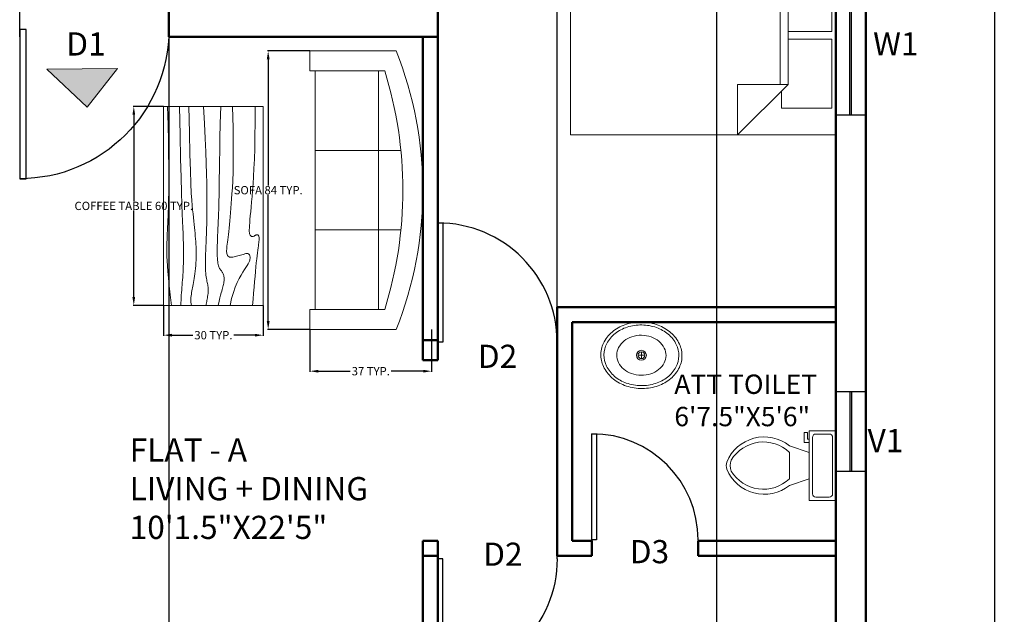
# Model space of a CAD drawing. Units: inches. Extents: x 227 to 711, y 218 to 1048.
# Tile 3 of 5: x 414 to 711, y 411 to 590. Entities that reach past the tile are written whole.
import ezdxf

# ---------------------------------------------------------------- set-up
doc = ezdxf.new("R2010")
doc.units = ezdxf.units.IN
doc.header["$MEASUREMENT"] = 0
for name, color, linetype, lineweight in [('A-ANNO-DIMS', 2, 'Continuous', 18), ('A-ANNO-SYMB', 85, 'Continuous', 18), ('A-ANNO-TEXT', 70, 'Continuous', 18), ('A-AREA-IDEN', 70, 'Continuous', 25), ('A-FLOR-FIXT', 140, 'Continuous', 18), ('A-FURN', 8, 'Continuous', 18), ('A-WALL', 10, 'Continuous', 50), ('DOORS', 30, 'Continuous', 25), ('WINDOWS', 50, 'Continuous', 25)]:
    doc.layers.add(name, color=color, linetype=linetype, lineweight=lineweight)
doc.styles.get("Standard").update_dxf_attribs({"font": 'arial.ttf'})
doc.dimstyles.get("Standard").update_dxf_attribs({"dimtxt": 2.5, "dimasz": 2.5, "dimexe": 0.18, "dimexo": 0.0625, "dimgap": 0.09, "dimtad": 0, "dimtih": 1, "dimtoh": 1, "dimzin": 0, "dimdsep": 46, "dimlunit": 3, "dimtxsty": 'Standard', "dimcen": 0.09, "dimadec": 0, "dimazin": 0, "dimtfac": 1, "dimtofl": 0, "dimtmove": 0, "dimatfit": 3, "dimfxl": 1, "dimtolj": 1, "dimtzin": 0, "dimarcsym": 0})

# ---------------------------------------------------------------- blocks, each defined once
blk = doc.blocks.new('*U2')
for p, q in [((0, 0), (0, -6)), ((40, 0), (40, -6))]:
    blk.add_line(p, q)
blk.add_lwpolyline([(0, 0), (0, 40), (1.75, 40), (1.75, 0)], close=True)
blk.add_arc((0, 0), 40, 0, 90)
blk = doc.blocks.new('Bed - Queen')
for p, q in [((0, -80.00003), (0, 0)), ((0, 0), (59.99999, 0)), ((59.99999, 0), (59.99999, -80.00003)), ((7.99999, -1.2), (28.79998, -1.2)), ((7.99999, -14.4), (7.99999, -1.2)), ((28.79998, -1.2), (28.79998, -14.4)), ((31.19999, -1.2), (51.99999, -1.2)), ((31.19999, -14.4), (31.19999, -1.2)), ((51.99999, -1.2), (51.99999, -16.4)), ((0, -14.4), (44.8, -14.4)), ((59.99999, -29.6), (44.8, -14.4)), ((44.8, -14.4), (44.8, -29.6)), ((44.8, -16.8), (0, -16.8)), ((51.99999, -16.4), (46.79936, -16.4)), ((44.8, -29.6), (59.99999, -29.6)), ((59.99999, -80.00003), (0, -80.00003))]:
    blk.add_line(p, q)
blk = doc.blocks.new('Toilet - top')
for p, q in [((9.5, -6), (9.5, -2)), ((-10, -8.5), (-8, -8.5)), ((-10, -9.5), (-10, -8.5)), ((-8, -8.5), (-8, -8)), ((-7, -8), (-7, -9.5)), ((-4, -8), (-6, -14)), ((4, -8), (6, -14)), ((-7, -9.5), (-10, -9.5)), ((4, -14), (-4, -14))]:
    blk.add_line(p, q)
blk.add_lwpolyline([(10.5, -8), (10.5, 0), (-10.5, 0), (-10.5, -8)], close=True)
for points in [[(-9.5, -2), (-9.5, -6)], [(8.5, -1), (-8.5, -1)], [(-8.5, -7), (8.5, -7)]]:
    blk.add_lwpolyline(points)
for centre, radius, start, end in [((-8.62, -1.88), 0.884, 81.8699, 188.1301), ((8.62, -1.88), 0.884, 351.8699, 98.1301), ((-8.62, -6.12), 0.884, 171.8699, 278.1301), ((8.62, -6.12), 0.884, 261.8699, 8.1301), ((3.52, -21.58), 12.17, 141.4691, 247.9714), ((4.2, -21.82), 11.33, 136.3677, 238.9468), ((-3.52, -21.58), 12.17, 292.0284, 38.5307), ((-4.2, -21.82), 11.33, 301.053, 43.6321), ((0, -27.88), 4, 245.7318, 294.2682), ((0, -29), 4, 254.8605, 285.1395)]:
    blk.add_arc(centre, radius, start, end)
blk = doc.blocks.new('Sink - Oval top')
for p, q in [((-1, 0), (1, 0)), ((0, 1), (0, -1))]:
    blk.add_line(p, q)
for points in [[(-12.23, 0.39, 0.117634), (-11.46, -3.36, 0.104469), (-8.88, -6.8, 0.090016), (-5.08, -9.07, 0.08192), (-0.32, -10.02, 0.08192), (4.49, -9.38, 0.090016), (8.42, -7.36, 0.104469), (11.22, -4.09, 0.117634), (12.23, -0.39, 0.117634), (11.46, 3.36, 0.104469), (8.88, 6.8, 0.090016), (5.08, 9.07, 0.08192), (0.32, 10.02, 0.08192), (-4.49, 9.38, 0.090016), (-8.42, 7.36, 0.104469), (-11.22, 4.09, 0.117634)], [(-11.29, 0.16, 0.118622), (-10.52, -3.25, 0.104678), (-8.07, -6.36, 0.089562), (-4.54, -8.37, 0.081185), (-0.13, -9.15, 0.081185), (4.3, -8.49, 0.089562), (7.89, -6.58, 0.104678), (10.42, -3.55, 0.118622), (11.29, -0.16, 0.118622), (10.52, 3.25, 0.104678), (8.07, 6.36, 0.089562), (4.54, 8.37, 0.081185), (0.13, 9.15, 0.081185), (-4.3, 8.49, 0.089562), (-7.89, 6.58, 0.104678), (-10.42, 3.55, 0.118622)], [(-7.42, 0.08, 0.118283), (-6.91, -2.17, 0.104607), (-5.29, -4.21, 0.089718), (-2.97, -5.53, 0.081436), (-0.07, -6.04, 0.081436), (2.84, -5.59, 0.089718), (5.2, -4.33, 0.104607), (6.86, -2.32, 0.118283), (7.42, -0.08, 0.118283), (6.91, 2.17, 0.104607), (5.29, 4.21, 0.089718), (2.97, 5.53, 0.081436), (0.07, 6.04, 0.081436), (-2.84, 5.59, 0.089718), (-5.2, 4.33, 0.104607), (-6.86, 2.32, 0.118283)]]:
    blk.add_lwpolyline(points, format="xyb", close=True)
for radius in [1.5, 1]:
    blk.add_circle((0, 0), radius)
blk = doc.blocks.new('Sofa - Roundback 7 ft.')
for p, q in [((-12.00002, -32.4421), (-12.00003, -6.5971)), ((11.99997, -32.4421), (11.99998, -6.5971)), ((-36.000027, -34), (-36.000027, -11.4696)), ((35.99998, -34), (35.99998, -11.4696)), ((-35.999844, -13.3819), (35.9998, -13.3819)), ((-36.000027, -32.4421), (35.99998, -32.4421))]:
    blk.add_line(p, q)
for points in [[(-36.000027, -34), (-42.000027, -34), (-42.000027, -8)], [(41.99998, -8), (41.99998, -34), (35.99998, -34)]]:
    blk.add_lwpolyline(points)
for centre, radius, start, end in [((0, -114.25), 114.25, 68.43141, 111.5686), ((-0.00001, -127.1968), 121.1968, 72.72033, 107.2797)]:
    blk.add_arc(centre, radius, start, end)
blk = doc.blocks.new('Table - Rectangular Woodgrain 60 x 30 in.')
for p, q in [((0, 0), (0, -30)), ((60, 0), (0, 0)), ((60, -30), (60, 0)), ((0, -30), (60, -30))]:
    blk.add_line(p, q)
for points in [[(0, -2.4), (4.8155, -2.418), (9.0302, -2.4688), (12.709, -2.5477), (15.9167, -2.65), (18.7181, -2.7711), (21.1781, -2.9063), (23.3616, -3.0508), (25.3333, -3.2), (27.1477, -3.3495), (28.8172, -3.4958), (30.3437, -3.636), (31.7291, -3.7667), (32.9756, -3.8849), (34.0849, -3.9875), (35.059, -4.0714), (35.9, -4.1334), (36.6114, -4.1711), (37.2041, -4.1854), (37.6906, -4.1779), (38.0833, -4.15), (38.3948, -4.1034), (38.6375, -4.0396), (38.8239, -3.9602), (38.9666, -3.8667), (39.0764, -3.7608), (39.1573, -3.6448), (39.2116, -3.521), (39.2416, -3.3917), (39.2498, -3.2593), (39.2385, -3.1261), (39.21, -2.9944), (39.1666, -2.8667), (39.111, -2.7447), (39.0468, -2.6281), (38.978, -2.5163), (38.9083, -2.4083), (38.8418, -2.3035), (38.7823, -2.201), (38.7337, -2.1001), (38.7, -2), (38.6844, -1.9003), (38.6875, -1.8021), (38.7094, -1.707), (38.75, -1.6167), (38.8094, -1.5326), (38.8875, -1.4563), (38.9844, -1.3893), (39.1, -1.3333), (39.2351, -1.2896), (39.3937, -1.2583), (39.5804, -1.2396), (39.8, -1.2333), (40.057, -1.2396), (40.3562, -1.2583), (40.7023, -1.2896), (41.1, -1.3333), (41.5547, -1.3895), (42.0755, -1.4573), (42.6721, -1.5361), (43.3542, -1.625), (44.1316, -1.7233), (45.014, -1.8302), (46.0114, -1.9449), (47.1333, -2.0667), (48.3862, -2.1947), (49.7625, -2.3281), (51.2513, -2.4663), (52.8416, -2.6083), (54.5226, -2.7535), (56.2833, -2.9011), (58.1127, -3.0501), (60, -3.2)], [(0, -9.2), (6.5759, -9.0858), (11.9385, -9.0365), (16.2527, -9.0418), (19.6833, -9.0917), (22.3952, -9.1759), (24.5531, -9.2844), (26.322, -9.4069), (27.8666, -9.5333), (29.3241, -9.6553), (30.7203, -9.7719), (32.0532, -9.8837), (33.3208, -9.9917), (34.5213, -10.0965), (35.6526, -10.199), (36.7128, -10.2999), (37.7, -10.4), (38.6129, -10.4996), (39.4531, -10.5969), (40.223, -10.6895), (40.925, -10.775), (41.5613, -10.8512), (42.1344, -10.9156), (42.6465, -10.966), (43.1, -11), (43.4976, -11.0158), (43.8437, -11.0136), (44.143, -10.9942), (44.4, -10.9583), (44.6195, -10.9069), (44.8062, -10.8406), (44.9648, -10.7603), (45.1, -10.6667), (45.2155, -10.5598), (45.3114, -10.4365), (45.3871, -10.2929), (45.4416, -10.125), (45.4743, -9.929), (45.4844, -9.7011), (45.4709, -9.4371), (45.4333, -9.1333), (45.3716, -8.7883), (45.2896, -8.4104), (45.1919, -8.0107), (45.0833, -7.6), (44.9685, -7.1893), (44.8521, -6.7896), (44.7388, -6.4117), (44.6333, -6.0667), (44.54, -5.7628), (44.4614, -5.4979), (44.4001, -5.2675), (44.3583, -5.0667), (44.3384, -4.8909), (44.3427, -4.7354), (44.3736, -4.5956), (44.4333, -4.4667), (44.5236, -4.3453), (44.6427, -4.2333), (44.7884, -4.1339), (44.9583, -4.05), (45.1501, -3.9849), (45.3614, -3.9417), (45.59, -3.9234), (45.8333, -3.9333), (46.0915, -3.9749), (46.3734, -4.0531), (46.6906, -4.1736), (47.0542, -4.3417), (47.4756, -4.5629), (47.9661, -4.8427), (48.5372, -5.1866), (49.2, -5.6), (49.9676, -6.0844), (50.8594, -6.625), (51.8965, -7.2031), (53.1, -7.8), (54.491, -8.3969), (56.0906, -8.975), (57.9199, -9.5156), (60, -10)], [(0, -12.8), (5.1847, -12.9322), (9.6213, -13.0323), (13.3963, -13.1059), (16.5958, -13.1583), (19.3063, -13.1952), (21.614, -13.2219), (23.6054, -13.2439), (25.3666, -13.2667), (26.9728, -13.2947), (28.4531, -13.3281), (29.8256, -13.3663), (31.1083, -13.4083), (32.3191, -13.4535), (33.476, -13.501), (34.597, -13.5501), (35.7, -13.6), (36.7984, -13.6497), (37.8875, -13.6979), (38.9578, -13.743), (40, -13.7833), (41.0047, -13.8174), (41.9625, -13.8438), (42.864, -13.8607), (43.7, -13.8667), (44.4631, -13.8604), (45.1552, -13.8417), (45.7801, -13.8104), (46.3416, -13.7667), (46.8439, -13.7104), (47.2906, -13.6417), (47.6858, -13.5604), (48.0333, -13.4667), (48.3375, -13.3608), (48.6042, -13.2448), (48.8396, -13.121), (49.05, -12.9917), (49.2417, -12.8593), (49.4208, -12.7261), (49.5937, -12.5944), (49.7667, -12.4667), (49.9452, -12.3451), (50.1323, -12.2313), (50.3303, -12.1268), (50.5416, -12.0333), (50.7686, -11.9524), (51.0135, -11.8854), (51.2788, -11.8341), (51.5666, -11.8), (51.8785, -11.7843), (52.2116, -11.7865), (52.562, -11.8059), (52.926, -11.8417), (53.2998, -11.8931), (53.6795, -11.9594), (54.0614, -12.0397), (54.4416, -12.1333), (54.8223, -12.2401), (55.2293, -12.3625), (55.6942, -12.5037), (56.2489, -12.6667), (56.9251, -12.8547), (57.7545, -13.0708), (58.7689, -13.3182), (60, -13.6)], [(0, -18), (5.124, -17.7273), (9.6609, -17.5057), (13.6705, -17.3303), (17.2125, -17.1958), (20.3467, -17.0973), (23.1328, -17.0297), (25.6307, -16.9878), (27.9, -16.9667), (29.9928, -16.9617), (31.9302, -16.9703), (33.7254, -16.9907), (35.3917, -17.0208), (36.9423, -17.0588), (38.3906, -17.1026), (39.7499, -17.1503), (41.0333, -17.2), (42.2519, -17.2496), (43.4073, -17.2969), (44.4986, -17.3395), (45.525, -17.375), (46.4858, -17.4012), (47.3802, -17.4156), (48.2074, -17.416), (48.9667, -17.4), (49.6583, -17.3662), (50.2872, -17.3167), (50.8595, -17.2547), (51.3812, -17.1833), (51.8584, -17.1057), (52.2971, -17.025), (52.7034, -16.9443), (53.0833, -16.8667), (53.443, -16.7951), (53.789, -16.7313), (54.128, -16.6768), (54.4666, -16.6334), (54.8115, -16.6024), (55.1693, -16.5854), (55.5465, -16.5841), (55.95, -16.6), (56.3828, -16.6337), (56.8346, -16.6823), (57.2915, -16.7418), (57.7396, -16.8084), (58.165, -16.878), (58.5539, -16.9469), (58.8924, -17.0111), (59.1666, -17.0667), (59.3679, -17.1107), (59.5078, -17.1438), (59.6032, -17.1675), (59.6708, -17.1833), (59.7275, -17.193), (59.7901, -17.1979), (59.8753, -17.1998), (60, -17.2)], [(0, -22.4), (8.0098, -22.2501), (14.4094, -22.1011), (19.4168, -21.9535), (23.25, -21.8083), (26.1269, -21.6663), (28.2656, -21.5281), (29.884, -21.3947), (31.2, -21.2667), (32.3967, -21.1448), (33.5172, -21.0292), (34.5697, -20.9198), (35.5625, -20.8167), (36.5037, -20.7198), (37.4015, -20.6292), (38.2642, -20.5448), (39.1, -20.4667), (39.9164, -20.3951), (40.7187, -20.3313), (41.5117, -20.2768), (42.3, -20.2333), (43.0883, -20.2024), (43.8812, -20.1854), (44.6836, -20.1841), (45.5, -20.2), (46.3328, -20.234), (47.1747, -20.2844), (48.0163, -20.3488), (48.8479, -20.425), (49.66, -20.5106), (50.4429, -20.6031), (51.1872, -20.7004), (51.8833, -20.8), (52.5246, -20.8999), (53.1166, -20.9995), (53.6681, -21.0983), (54.1875, -21.1958), (54.6834, -21.2919), (55.1646, -21.3859), (55.6394, -21.4777), (56.1167, -21.5667), (56.6028, -21.6515), (57.0961, -21.7266), (57.5929, -21.7852), (58.0896, -21.8208), (58.5823, -21.8268), (59.0674, -21.7964), (59.5412, -21.723), (60, -21.6)], [(0, -25.2), (8.6355, -25.0504), (15.7026, -24.9031), (21.4049, -24.7606), (25.9458, -24.625), (29.529, -24.4988), (32.3578, -24.3844), (34.6359, -24.284), (36.5667, -24.2), (38.3213, -24.1341), (39.9417, -24.0854), (41.437, -24.0523), (42.8167, -24.0333), (44.0901, -24.0268), (45.2667, -24.0313), (46.3557, -24.0451), (47.3667, -24.0667), (48.309, -24.0947), (49.1928, -24.1287), (50.0284, -24.168), (50.826, -24.2125), (51.5959, -24.2617), (52.3483, -24.3151), (53.0935, -24.3725), (53.8417, -24.4334), (54.6009, -24.497), (55.3699, -24.561), (56.1454, -24.6226), (56.9239, -24.6792), (57.7021, -24.7279), (58.4764, -24.7662), (59.2435, -24.7911), (60, -24.8)], [(0, -28.8), (5.6867, -28.6681), (10.45, -28.5698), (14.407, -28.5012), (17.675, -28.4584), (20.3711, -28.4374), (22.6125, -28.4344), (24.5164, -28.4455), (26.2, -28.4667), (27.762, -28.4947), (29.2276, -28.5281), (30.6033, -28.5663), (31.8958, -28.6084), (33.1118, -28.6535), (34.2578, -28.7011), (35.3405, -28.7501), (36.3666, -28.8), (37.3443, -28.8497), (38.288, -28.8974), (39.2137, -28.9412), (40.1375, -28.9792), (41.0753, -29.0093), (42.0432, -29.0297), (43.0572, -29.0384), (44.1333, -29.0333), (45.2936, -29.0114), (46.5843, -28.9641), (48.0579, -28.8816), (49.7666, -28.7542), (51.7629, -28.5721), (54.0989, -28.3255), (56.8272, -28.0048), (60, -27.6)]]:
    blk.add_lwpolyline(points)
blk = doc.blocks.new('WIN-48IN')
for p, q in [((0, 4.75), (48, 4.75)), ((0, 4.25), (48, 4.25))]:
    blk.add_line(p, q)
blk.add_lwpolyline([(0, 0), (48, 0), (48, 9), (0, 9)], close=True)
blk = doc.blocks.new('VENT-V1-24IN')
for p, q in [((4.25, 24), (4.25, 0)), ((4.75, 24), (4.75, 0))]:
    blk.add_line(p, q)
blk.add_lwpolyline([(0, 24), (0, 0), (9, 0), (9, 24)], close=True)
blk = doc.blocks.new('ENTRY-DIRECTION')
h = blk.add_hatch(color=256)
h.dxf.hatch_style = 1
h.paths.add_polyline_path([(21.25, 11.69), (0, 11.44), (12.11, 0)])
for p, q in [((21.25, 11.69), (0, 11.44)), ((0, 11.44), (12.11, 0)), ((12.11, 0), (21.25, 11.69))]:
    blk.add_line(p, q)
blk = doc.blocks.new('*D34')
at = {"layer": 'A-ANNO-DIMS', "color": 0, "lineweight": -2, "transparency": 16777216}
for p, q in [((501.93, 580.85), (489.21, 580.85)), ((489.39, 578.35), (489.39, 540.23)), ((489.39, 499.35), (489.39, 537.46)), ((501.93, 496.85), (489.21, 496.85))]:
    blk.add_line(p, q, dxfattribs=at)
at = {"layer": 'A-ANNO-DIMS', "color": 0, "transparency": 16777216}
for points in [[(488.97, 578.35), (489.81, 578.35), (489.39, 580.85)], [(488.97, 499.35), (489.81, 499.35), (489.39, 496.85)]]:
    blk.add_solid(points, dxfattribs=at)
at = {"layer": 'Defpoints', "color": 0, "transparency": 16777216}
for p in [(501.99, 580.85), (489.39, 496.85), (501.99, 496.85)]:
    blk.add_point(p, dxfattribs=at)
at = {"layer": 'A-ANNO-DIMS', "color": 0, "transparency": 16777216, "insert": (489.39, 538.85), "char_height": 2.5, "attachment_point": 5}
blk.add_mtext('\\A1;SOFA 84 TYP.', dxfattribs=at)
blk = doc.blocks.new('*D35')
at = {"layer": 'A-ANNO-DIMS', "color": 0, "lineweight": -2, "transparency": 16777216}
for p, q in [((501.99, 496.78), (501.99, 484.07)), ((538.66, 496.78), (538.66, 484.07)), ((504.49, 484.25), (514.15, 484.25)), ((536.16, 484.25), (526.5, 484.25))]:
    blk.add_line(p, q, dxfattribs=at)
at = {"layer": 'A-ANNO-DIMS', "color": 0, "transparency": 16777216}
for points in [[(504.49, 484.66), (504.49, 483.83), (501.99, 484.25)], [(536.16, 484.66), (536.16, 483.83), (538.66, 484.25)]]:
    blk.add_solid(points, dxfattribs=at)
at = {"layer": 'Defpoints', "color": 0, "transparency": 16777216}
for p in [(501.99, 496.85), (538.66, 496.85), (538.66, 484.25)]:
    blk.add_point(p, dxfattribs=at)
at = {"layer": 'A-ANNO-DIMS', "color": 0, "transparency": 16777216, "insert": (520.32, 484.25), "char_height": 2.5, "attachment_point": 5}
blk.add_mtext('\\A1;37 TYP.', dxfattribs=at)
blk = doc.blocks.new('*D38')
at = {"layer": 'A-ANNO-DIMS', "color": 0, "lineweight": -2, "transparency": 16777216}
for p, q in [((457.82, 564.11), (448.7, 564.11)), ((448.88, 561.61), (448.88, 535.49)), ((448.88, 506.61), (448.88, 532.73)), ((457.82, 504.11), (448.7, 504.11))]:
    blk.add_line(p, q, dxfattribs=at)
at = {"layer": 'A-ANNO-DIMS', "color": 0, "transparency": 16777216}
for points in [[(448.47, 561.61), (449.3, 561.61), (448.88, 564.11)], [(448.47, 506.61), (449.3, 506.61), (448.88, 504.11)]]:
    blk.add_solid(points, dxfattribs=at)
at = {"layer": 'Defpoints', "color": 0, "transparency": 16777216}
for p in [(457.88, 564.11), (448.88, 504.11), (457.88, 504.11)]:
    blk.add_point(p, dxfattribs=at)
at = {"layer": 'A-ANNO-DIMS', "color": 0, "transparency": 16777216, "insert": (448.88, 534.11), "char_height": 2.5, "attachment_point": 5}
blk.add_mtext('\\A1;COFFEE TABLE 60 TYP.', dxfattribs=at)
blk = doc.blocks.new('*D39')
at = {"layer": 'A-ANNO-DIMS', "color": 0, "lineweight": -2, "transparency": 16777216}
for p, q in [((457.88, 504.05), (457.88, 494.93)), ((487.88, 504.05), (487.88, 494.93)), ((460.38, 495.11), (466.71, 495.11)), ((485.38, 495.11), (479.06, 495.11))]:
    blk.add_line(p, q, dxfattribs=at)
at = {"layer": 'A-ANNO-DIMS', "color": 0, "transparency": 16777216}
for points in [[(460.38, 495.53), (460.38, 494.69), (457.88, 495.11)], [(485.38, 495.53), (485.38, 494.69), (487.88, 495.11)]]:
    blk.add_solid(points, dxfattribs=at)
at = {"layer": 'Defpoints', "color": 0, "transparency": 16777216}
for p in [(457.88, 504.11), (487.88, 504.11), (487.88, 495.11)]:
    blk.add_point(p, dxfattribs=at)
at = {"layer": 'A-ANNO-DIMS', "color": 0, "transparency": 16777216, "insert": (472.88, 495.11), "char_height": 2.5, "attachment_point": 5}
blk.add_mtext('\\A1;30 TYP.', dxfattribs=at)
blk = doc.blocks.new('*D45')
at = {"layer": 'A-ANNO-DIMS', "color": 0, "lineweight": -2, "transparency": 16777216}
for p, q in [((669.55, 1007.07), (708.62, 1007.07)), ((708.44, 1004.57), (708.44, 634.43)), ((708.44, 261.57), (708.44, 631.7)), ((669.55, 259.07), (708.62, 259.07))]:
    blk.add_line(p, q, dxfattribs=at)
at = {"layer": 'A-ANNO-DIMS', "color": 0, "transparency": 16777216}
for points in [[(708.02, 1004.57), (708.86, 1004.57), (708.44, 1007.07)], [(708.02, 261.57), (708.86, 261.57), (708.44, 259.07)]]:
    blk.add_solid(points, dxfattribs=at)
at = {"layer": 'Defpoints', "color": 0, "transparency": 16777216}
for p in [(669.49, 1007.07), (708.44, 1007.07), (669.49, 259.07)]:
    blk.add_point(p, dxfattribs=at)
at = {"layer": 'A-ANNO-DIMS', "color": 0, "transparency": 16777216, "insert": (708.44, 633.07), "char_height": 2.5, "attachment_point": 5}
blk.add_mtext('\\A1;748', dxfattribs=at)
blk = doc.blocks.new('*D53')
at = {"layer": 'A-ANNO-DIMS', "color": 0, "lineweight": -2, "transparency": 16777216}
for p, q in [((414.49, 585.13), (414.49, 1046.2)), ((416.99, 1046.02), (435.05, 1046.02)), ((456.99, 1046.02), (438.93, 1046.02)), ((459.49, 585.13), (459.49, 1046.2))]:
    blk.add_line(p, q, dxfattribs=at)
at = {"layer": 'A-ANNO-DIMS', "color": 0, "transparency": 16777216}
for points in [[(416.99, 1046.43), (416.99, 1045.6), (414.49, 1046.02)], [(456.99, 1046.43), (456.99, 1045.6), (459.49, 1046.02)]]:
    blk.add_solid(points, dxfattribs=at)
at = {"layer": 'Defpoints', "color": 0, "transparency": 16777216}
for p in [(459.49, 1046.02), (414.49, 585.07), (459.49, 585.07)]:
    blk.add_point(p, dxfattribs=at)
at = {"layer": 'A-ANNO-DIMS', "color": 0, "transparency": 16777216, "insert": (436.99, 1046.02), "char_height": 2.5, "attachment_point": 5}
blk.add_mtext('\\A1;45', dxfattribs=at)
blk = doc.blocks.new('*D56')
at = {"layer": 'A-ANNO-DIMS', "color": 0, "lineweight": -2, "transparency": 16777216}
for p, q in [((540.49, 493.63), (540.49, 1046.2)), ((542.99, 1046.02), (556.61, 1046.02)), ((573.99, 1046.02), (560.37, 1046.02)), ((576.49, 493.03), (576.49, 1046.2))]:
    blk.add_line(p, q, dxfattribs=at)
at = {"layer": 'A-ANNO-DIMS', "color": 0, "transparency": 16777216}
for points in [[(542.99, 1046.43), (542.99, 1045.6), (540.49, 1046.02)], [(573.99, 1046.43), (573.99, 1045.6), (576.49, 1046.02)]]:
    blk.add_solid(points, dxfattribs=at)
at = {"layer": 'Defpoints', "color": 0, "transparency": 16777216}
for p in [(576.49, 1046.02), (540.49, 493.57), (576.49, 492.97)]:
    blk.add_point(p, dxfattribs=at)
at = {"layer": 'A-ANNO-DIMS', "color": 0, "transparency": 16777216, "insert": (558.49, 1046.02), "char_height": 2.5, "attachment_point": 5}
blk.add_mtext('\\A1;36', dxfattribs=at)
blk = doc.blocks.new('*D60')
at = {"layer": 'A-ANNO-DIMS', "color": 0, "lineweight": -2, "transparency": 16777216}
for p, q in [((459.49, 681), (459.49, 219.94)), ((409.99, 636), (409.99, 219.94)), ((412.49, 220.12), (431.34, 220.12)), ((456.99, 220.12), (438.14, 220.12))]:
    blk.add_line(p, q, dxfattribs=at)
at = {"layer": 'A-ANNO-DIMS', "color": 0, "transparency": 16777216}
for points in [[(412.49, 220.53), (412.49, 219.7), (409.99, 220.12)], [(456.99, 220.53), (456.99, 219.7), (459.49, 220.12)]]:
    blk.add_solid(points, dxfattribs=at)
at = {"layer": 'Defpoints', "color": 0, "transparency": 16777216}
for p in [(459.49, 681.07), (409.99, 636.07), (459.49, 220.12)]:
    blk.add_point(p, dxfattribs=at)
at = {"layer": 'A-ANNO-DIMS', "color": 0, "transparency": 16777216, "insert": (434.74, 220.12), "char_height": 2.5, "attachment_point": 5}
blk.add_mtext('\\A1;49.5', dxfattribs=at)
blk = doc.blocks.new('*D62')
at = {"layer": 'A-ANNO-DIMS', "color": 0, "lineweight": -2, "transparency": 16777216}
for p, q in [((624.49, 998), (624.49, 219.94)), ((660.49, 998), (660.49, 219.94)), ((626.99, 220.12), (640.61, 220.12)), ((657.99, 220.12), (644.37, 220.12))]:
    blk.add_line(p, q, dxfattribs=at)
at = {"layer": 'A-ANNO-DIMS', "color": 0, "transparency": 16777216}
for points in [[(626.99, 220.53), (626.99, 219.7), (624.49, 220.12)], [(657.99, 220.53), (657.99, 219.7), (660.49, 220.12)]]:
    blk.add_solid(points, dxfattribs=at)
at = {"layer": 'Defpoints', "color": 0, "transparency": 16777216}
for p in [(624.49, 998.07), (660.49, 998.07), (660.49, 220.12)]:
    blk.add_point(p, dxfattribs=at)
at = {"layer": 'A-ANNO-DIMS', "color": 0, "transparency": 16777216, "insert": (642.49, 220.12), "char_height": 2.5, "attachment_point": 5}
blk.add_mtext('\\A1;36', dxfattribs=at)

msp = doc.modelspace()

# ---------------------------------------------------------------- linework, layer by layer
at = {"layer": 'A-WALL'}
for p, q in [((660.49, 499.065), (660.49, 672.065)), ((540.49, 585.065), (459.49, 585.065)), ((535.99, 585.065), (535.99, 565.565)), ((540.49, 585.065), (540.49, 487.572)), ((535.99, 565.565), (535.99, 487.572)), ((660.49, 503.565), (576.49, 503.565)), ((576.49, 428.565), (576.49, 503.565)), ((660.49, 499.065), (580.99, 499.065)), ((580.99, 433.065), (580.99, 499.065)), ((660.49, 433.065), (660.49, 499.065)), ((540.49, 493.572), (535.99, 493.572)), ((535.99, 493.572), (535.99, 487.572)), ((540.49, 487.572), (540.49, 493.572)), ((535.99, 487.572), (540.49, 487.572)), ((540.49, 433.065), (535.99, 433.065)), ((535.99, 433.065), (535.99, 325.065)), ((540.49, 433.065), (540.49, 428.565)), ((540.49, 433.065), (540.49, 268.065)), ((586.99, 433.065), (580.99, 433.065)), ((586.99, 428.565), (586.99, 433.065)), ((660.49, 433.065), (618.99, 433.065)), ((618.99, 428.565), (618.99, 433.065)), ((660.49, 268.065), (660.49, 433.065)), ((535.99, 428.565), (540.49, 428.565)), ((540.49, 428.565), (535.99, 428.565)), ((586.99, 428.565), (576.49, 428.565)), ((660.49, 428.565), (618.99, 428.565))]:
    msp.add_line(p, q, dxfattribs=at)
for points in [[(535.99, 259.065), (669.49, 259.065), (669.49, 1007.065), (535.99, 1007.065)], [(459.49, 681.226), (459.49, 652.565), (459.49, 585.065)], [(540.49, 681.226), (540.49, 652.565), (540.49, 585.065)]]:
    msp.add_lwpolyline(points, dxfattribs=at)

# ---------------------------------------------------------------- block references
at = {"layer": 'A-ANNO-SYMB'}
msp.add_blockref('ENTRY-DIRECTION', (422.71, 563.877), dxfattribs=at)
at = {"layer": 'A-FLOR-FIXT'}
msp.add_blockref('Sink - Oval top', (601.885, 489.049), dxfattribs=at)
at = {"layer": 'A-FLOR-FIXT', "rotation": 270}
msp.add_blockref('Toilet - top', (660.49, 455.767), dxfattribs=at)
at = {"layer": 'A-FURN', "rotation": 270}
for name, p in [('Bed - Queen', (660.49, 615.565)), ('Sofa - Roundback 7 ft.', (535.99, 538.846)), ('Table - Rectangular Woodgrain 60 x 30 in.', (487.885, 564.109))]:
    msp.add_blockref(name, p, dxfattribs=at)
at = {"layer": 'DOORS', "rotation": 180}
for p, xscale, yscale, zscale in [((414.49, 587.314), -1.12510570773799, 1.12510570773799, 1.12510570773799), ((540.49, 427.665), -0.9000000000000039, 0.9000000000000039, 0.9000000000000039)]:
    msp.add_blockref('*U2', p, dxfattribs=dict(at, xscale=xscale, yscale=yscale, zscale=zscale))
at = {"layer": 'DOORS'}
for p, xscale, yscale, zscale in [((540.49, 492.972), 0.9000000000000028, 0.9000000000000028, 0.9000000000000028), ((586.99, 433.365), 0.8, 0.8, 0.8)]:
    msp.add_blockref('*U2', p, dxfattribs=dict(at, xscale=xscale, yscale=yscale, zscale=zscale))
at = {"layer": 'WINDOWS', "rotation": 89.99999999999979}
msp.add_blockref('WIN-48IN', (669.49, 561.565), dxfattribs=at)
at = {"layer": 'WINDOWS'}
msp.add_blockref('VENT-V1-24IN', (660.49, 454.065), dxfattribs=at)

# ---------------------------------------------------------------- texts
at = {"layer": 'A-ANNO-TEXT', "char_height": 7, "attachment_point": 1}
for s, insert in [('D1', (428.526, 586.456)), ('W1', (671.731, 586.498)), ('D2', (552.585, 492.225)), ('V1', (670.072, 466.82)), ('D3', (598.376, 433.314)), ('D2', (554.209, 432.539))]:
    msp.add_mtext_dynamic_manual_height_columns(s, width=74.58955, gutter_width=1, heights=[0], dxfattribs=dict(at, insert=insert))
at = {"layer": 'A-AREA-IDEN', "attachment_point": 1}
for s, width, gutter_width, insert, char_height in [('ATT TOILET\\P6\'7.5"X5\'6"', 62.30128, 0.835, (611.817, 483.241), 5.84678), ('FLAT - A\\PLIVING + DINING\\P10\'1.5"X22\'5"', 78.17409, 1, (447.634, 463.981), 7)]:
    msp.add_mtext_dynamic_manual_height_columns(s, width=width, gutter_width=gutter_width, heights=[0], dxfattribs=dict(at, insert=insert, char_height=char_height))

# ---------------------------------------------------------------- dimensions: what is measured, and where the dimension line sits
at = {"layer": 'A-ANNO-DIMS'}
for base, p1, p2, override, picture, middle in [((459.49, 1046.015), (414.49, 585.065), (459.49, 585.065), {"dimdec": 0, "dimlfac": 1, "dimrnd": 0, "dimzin": 0, "dimdsep": 46, "dimlunit": 2}, '*D53', (436.99, 1046.015)), ((576.49, 1046.015), (540.49, 493.572), (576.49, 492.972), {"dimdec": 0, "dimlfac": 1, "dimrnd": 0, "dimzin": 0, "dimdsep": 46, "dimlunit": 2}, '*D56', (558.49, 1046.015)), ((660.49, 220.115), (624.49, 998.065), (660.49, 998.065), {"dimdec": 0, "dimlfac": 1, "dimrnd": 0, "dimzin": 0, "dimdsep": 46, "dimlunit": 2}, '*D62', (642.49, 220.115)), ((459.49, 220.115), (409.99, 636.065), (459.49, 681.065), {"dimdec": 1, "dimlfac": 1, "dimrnd": 0, "dimzin": 0, "dimdsep": 46, "dimlunit": 2}, '*D60', (434.74, 220.115))]:
    dim = msp.add_linear_dim(base=base, p1=p1, p2=p2, dimstyle='Standard', override=override, dxfattribs=at)
    dim.commit()
    dim.dimension.update_dxf_attribs({"geometry": picture, "text_midpoint": middle})
dim = msp.add_linear_dim(base=(708.44, 1007.065), p1=(669.49, 259.065), p2=(669.49, 1007.065), angle=90, dimstyle='Standard', override={"dimdec": 0, "dimlfac": 1, "dimrnd": 0, "dimzin": 0, "dimdsep": 46, "dimlunit": 2}, dxfattribs=at)
dim.commit()
dim.dimension.update_dxf_attribs({"geometry": '*D45', "text_midpoint": (708.44, 633.065)})
for base, p1, p2, text, picture, middle in [((489.39, 496.846), (501.99, 580.846), (501.99, 496.846), 'SOFA <> TYP.', '*D34', (489.39, 538.846)), ((448.885, 504.109), (457.885, 564.109), (457.885, 504.109), 'COFFEE TABLE <> TYP.', '*D38', (448.885, 534.109))]:
    dim = msp.add_linear_dim(base=base, p1=p1, p2=p2, angle=270, text=text, dimstyle='Standard', override={"dimdec": 0, "dimlfac": 1, "dimrnd": 0, "dimzin": 0, "dimdsep": 46, "dimlunit": 2}, dxfattribs=at)
    dim.commit()
    dim.dimension.update_dxf_attribs({"geometry": picture, "text_midpoint": middle})
for base, p1, p2, picture, middle in [((487.885, 495.109), (457.885, 504.109), (487.885, 504.109), '*D39', (472.885, 495.109)), ((538.657, 484.246), (501.99, 496.846), (538.657, 496.846), '*D35', (520.323, 484.246))]:
    dim = msp.add_linear_dim(base=base, p1=p1, p2=p2, text='<> TYP.', dimstyle='Standard', override={"dimdec": 0, "dimlfac": 1, "dimrnd": 0, "dimzin": 0, "dimdsep": 46, "dimlunit": 2}, dxfattribs=at)
    dim.commit()
    dim.dimension.update_dxf_attribs({"geometry": picture, "text_midpoint": middle})

doc.saveas('drawing.dxf')
